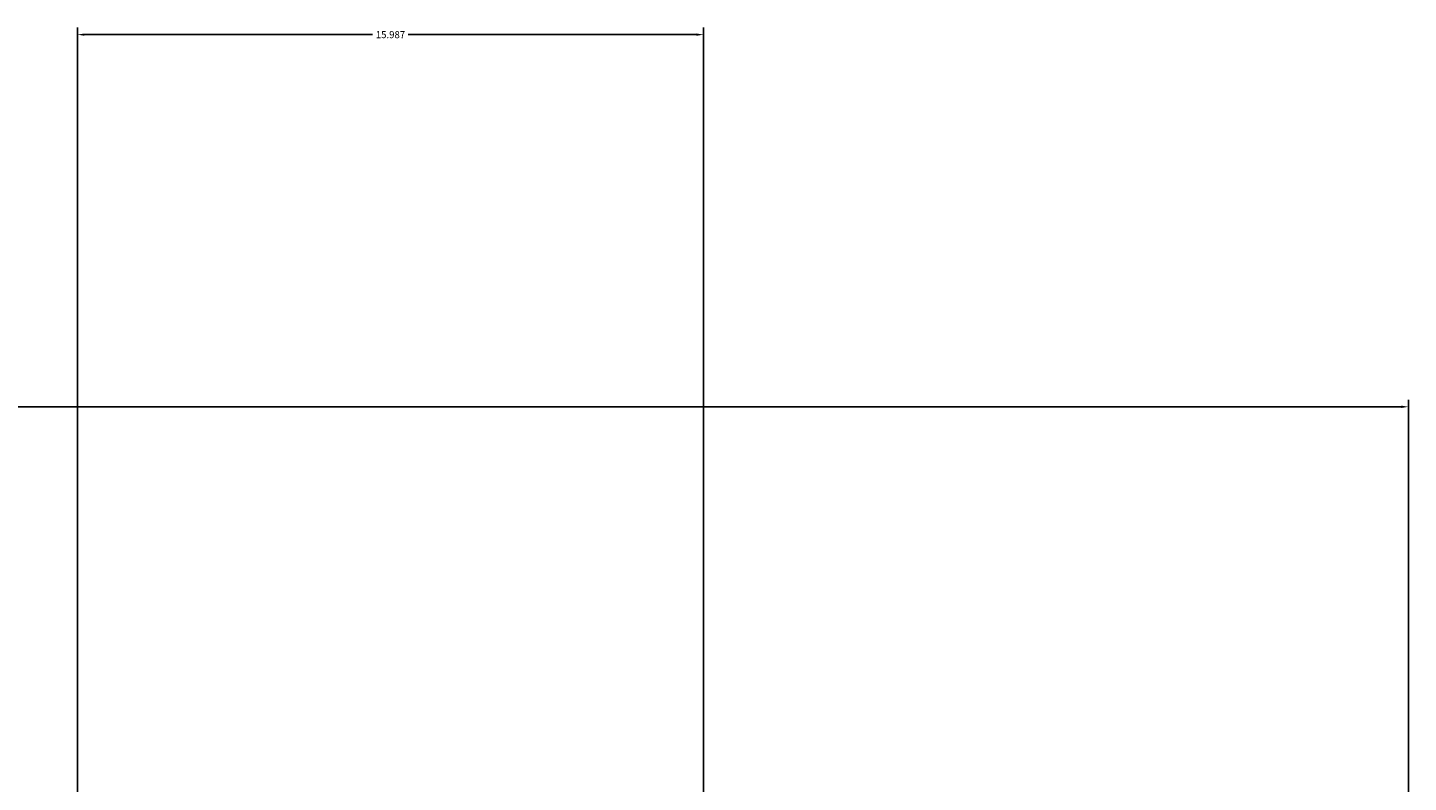
# Model space of a CAD drawing. Units: inches. Extents: x 2307 to 2544, y 2171 to 2540.
# Tile 29 of 52: x 2416 to 2452, y 2521 to 2540. Entities that reach past the tile are written whole.
import ezdxf

# ---------------------------------------------------------------- set-up
doc = ezdxf.new("R2010")
doc.units = ezdxf.units.IN
doc.layers.add('A-ANNO-DIMS', color=2, linetype='Continuous', lineweight=18)
doc.styles.get("Standard").update_dxf_attribs({"font": 'arial.ttf'})
doc.dimstyles.get("Standard").update_dxf_attribs({"dimtxt": 0.18, "dimasz": 0.18, "dimexe": 0.18, "dimexo": 0.0625, "dimgap": 0.09, "dimtad": 0, "dimtih": 1, "dimtoh": 1, "dimdec": 4, "dimzin": 0, "dimdsep": 46, "dimtxsty": 'Standard', "dimcen": 0.09, "dimadec": 0, "dimazin": 0, "dimtfac": 1, "dimtdec": 4, "dimtofl": 0, "dimtmove": 0, "dimatfit": 3, "dimfxl": 1, "dimtolj": 1, "dimtzin": 0, "dimarcsym": 0})

# ---------------------------------------------------------------- blocks, each defined once
blk = doc.blocks.new('*D45')
at = {"layer": 'A-ANNO-DIMS', "color": 0, "lineweight": -2, "transparency": 16777216}
for p, q in [((2335.696, 2511.572), (2335.696, 2530.84)), ((2335.876, 2530.66), (2393.416, 2530.66)), ((2451.516, 2530.66), (2393.976, 2530.66)), ((2451.696, 2511.572), (2451.696, 2530.84))]:
    blk.add_line(p, q, dxfattribs=at)
at = {"layer": 'A-ANNO-DIMS', "color": 0, "transparency": 16777216}
for points in [[(2335.876, 2530.69), (2335.876, 2530.63), (2335.696, 2530.66)], [(2451.516, 2530.69), (2451.516, 2530.63), (2451.696, 2530.66)]]:
    blk.add_solid(points, dxfattribs=at)
at = {"layer": 'Defpoints', "color": 0, "transparency": 16777216}
for p in [(2451.696, 2530.66), (2335.696, 2511.51), (2451.696, 2511.51)]:
    blk.add_point(p, dxfattribs=at)
at = {"layer": 'A-ANNO-DIMS', "color": 0, "transparency": 16777216, "insert": (2393.696, 2530.66), "char_height": 0.18, "attachment_point": 5}
blk.add_mtext('\\A1;116', dxfattribs=at)
blk = doc.blocks.new('*D69')
at = {"layer": 'A-ANNO-DIMS', "color": 0, "lineweight": -2, "transparency": 16777216}
for p, q in [((2417.708, 2490.237), (2417.708, 2540.345)), ((2417.888, 2540.165), (2425.247, 2540.165)), ((2433.516, 2540.165), (2426.157, 2540.165)), ((2433.696, 2511.572), (2433.696, 2540.345))]:
    blk.add_line(p, q, dxfattribs=at)
at = {"layer": 'A-ANNO-DIMS', "color": 0, "transparency": 16777216}
for points in [[(2417.888, 2540.195), (2417.888, 2540.135), (2417.708, 2540.165)], [(2433.516, 2540.195), (2433.516, 2540.135), (2433.696, 2540.165)]]:
    blk.add_solid(points, dxfattribs=at)
at = {"layer": 'Defpoints', "color": 0, "transparency": 16777216}
for p in [(2433.696, 2540.165), (2433.696, 2511.51), (2417.708, 2490.174)]:
    blk.add_point(p, dxfattribs=at)
at = {"layer": 'A-ANNO-DIMS', "color": 0, "transparency": 16777216, "insert": (2425.702, 2540.165), "char_height": 0.18, "attachment_point": 5}
blk.add_mtext('\\A1;15.987', dxfattribs=at)

msp = doc.modelspace()

# ---------------------------------------------------------------- dimensions: what is measured, and where the dimension line sits
at = {"layer": 'A-ANNO-DIMS'}
for base, p1, p2, override, picture, middle in [((2433.6958, 2540.1649), (2417.7084, 2490.1742), (2433.6958, 2511.5096), {"dimdec": 3, "dimlfac": 1, "dimrnd": 0, "dimzin": 0, "dimdsep": 46, "dimlunit": 2}, '*D69', (2425.7021, 2540.1649)), ((2451.6958, 2530.6596), (2335.6958, 2511.5096), (2451.6958, 2511.5096), {"dimdec": 0, "dimlfac": 1, "dimrnd": 0, "dimzin": 0, "dimdsep": 46, "dimlunit": 2}, '*D45', (2393.6958, 2530.6596))]:
    dim = msp.add_linear_dim(base=base, p1=p1, p2=p2, dimstyle='Standard', override=override, dxfattribs=at)
    dim.commit()
    dim.dimension.update_dxf_attribs({"geometry": picture, "text_midpoint": middle})

doc.saveas('drawing.dxf')
